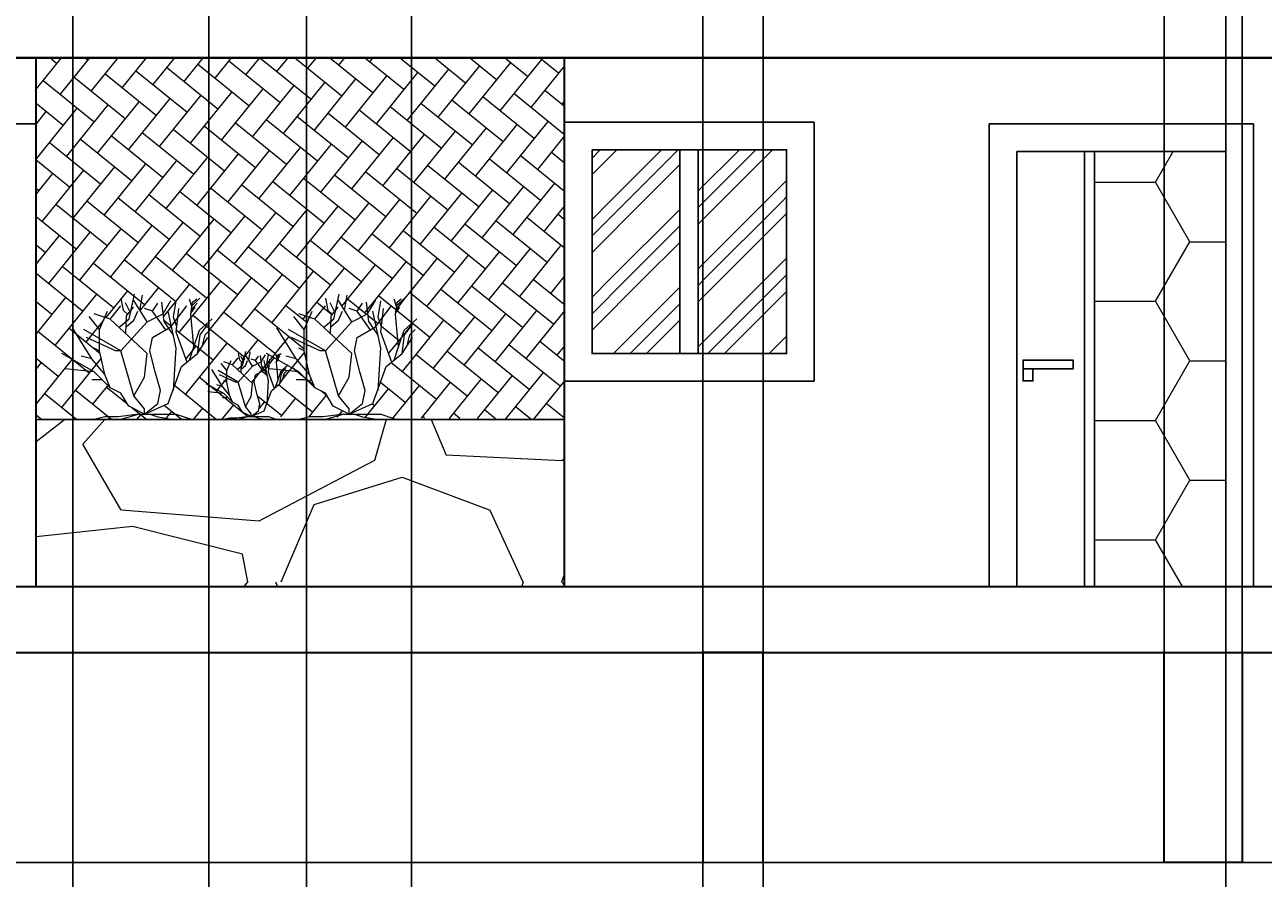
# Model space of a CAD drawing. Units: inches. Extents: x -8 to 554, y -200 to 499.
# Tile 4 of 12: x 214 to 439, y -34 to 121. Entities that reach past the tile are written whole.
import ezdxf

# ---------------------------------------------------------------- set-up
doc = ezdxf.new("R2010")
doc.units = ezdxf.units.IN
doc.header["$MEASUREMENT"] = 0
for name, color, linetype, lineweight in [('A-ANNO-DIMS', 2, 'Continuous', 18), ('A-COLS', 1, 'Continuous', 35), ('A-DOOR', 3, 'Continuous', 25), ('A-DOOR-GATE', 3, 'Continuous', 25), ('A-DOOR-PATT', 252, 'Continuous', 13), ('A-FLOR', 7, 'Continuous', 35), ('A-GLAZ', 4, 'Continuous', 25), ('A-GLAZ-PATT', 252, 'Continuous', 13), ('A-WALL', 7, 'Continuous', 35), ('A-WALL-PATT', 252, 'Continuous', 13), ('A-WALL-PRPT', 7, 'Continuous', 25), ('L-PLNT-TREE', 94, 'Continuous', 13)]:
    doc.layers.add(name, color=color, linetype=linetype, lineweight=lineweight)
doc.styles.get("Standard").update_dxf_attribs({"font": 'arial.ttf'})
doc.dimstyles.get("Standard").update_dxf_attribs({"dimtxt": 0.18, "dimasz": 0.18, "dimexe": 0.18, "dimexo": 0.0625, "dimgap": 0.09, "dimtad": 0, "dimtih": 1, "dimtoh": 1, "dimdec": 4, "dimzin": 0, "dimdsep": 46, "dimtxsty": 'Standard', "dimcen": 0.09, "dimadec": 0, "dimazin": 0, "dimtfac": 1, "dimtdec": 4, "dimtofl": 0, "dimtmove": 0, "dimatfit": 3, "dimfxl": 1, "dimtolj": 1, "dimtzin": 0, "dimarcsym": 0})

# ---------------------------------------------------------------- blocks, each defined once
blk = doc.blocks.new('*U2')
for p, q in [((-11.433, 18.289), (-10.457, 22.749)), ((-9.48, 19.775), (-8.992, 22.592)), ((-14.88, 18.24), (-12.96, 20.64)), ((-12.471, 19.775), (-12.898, 22.044)), ((-11.28, 19.619), (-12.104, 21.184)), ((-11.921, 18.836), (-10.64, 20.401)), ((-8.16, 17.76), (-10.56, 21.6)), ((-7.2, 19.68), (-6.24, 21.12)), ((-5.086, 17.741), (-5.513, 21.34)), ((-5.28, 19.2), (-3.84, 21.6)), ((-3.84, 16.8), (-0.96, 20.64)), ((-3.377, 18.602), (-2.888, 21.575)), ((-0.508, 21.888), (-0.081, 20.558)), ((-0.203, 19.149), (0.102, 21.34)), ((-0.142, 19.384), (0.59, 20.401)), ((-0.02, 20.01), (0.896, 21.105)), ((0.041, 20.714), (1.384, 22.044)), ((0.102, 21.34), (0.835, 21.888)), ((-16.8, 16.32), (-18.72, 18.72)), ((-14.88, 18.24), (-17.76, 19.2)), ((-16.8, 16.32), (-15.36, 19.68)), ((-8.16, 12), (-14.88, 18.24)), ((-13.325, 16.724), (-11.433, 18.289)), ((-11.677, 19.071), (-12.471, 19.775)), ((-12.043, 15.628), (-11.921, 18.836)), ((-11.982, 16.802), (-10.579, 18.054)), ((-10.579, 18.054), (-9.846, 19.697)), ((-7.2, 19.68), (-8.64, 20.16)), ((-8.16, 17.76), (-5.28, 19.2)), ((-4.8, 16.32), (-7.2, 19.68)), ((-2.88, 12.96), (-4.32, 19.68)), ((-2.766, 16.802), (-3.377, 18.602)), ((-2.88, 15.84), (-2.4, 20.16)), ((0.346, 13.203), (-0.203, 19.149)), ((1.323, 16.254), (3.642, 18.289)), ((-18.24, 11.04), (-21.755, 16.655)), ((-12.96, 12.48), (-19.68, 16.32)), ((-16.8, 12.48), (-16.8, 16.32)), ((-12.96, 12.48), (-8.16, 17.76)), ((-7.2, 14.88), (-3.84, 16.8)), ((-3.377, 15.315), (-5.086, 17.819)), ((-0.96, 10.56), (-2.88, 15.84)), ((0.346, 13.203), (1.323, 16.254)), ((1.44, 15.36), (2.88, 17.28)), ((2.4, 15.36), (3.36, 16.32)), ((-13.92, 12.48), (-19.2, 14.88)), ((-7.68, 12.48), (-7.2, 14.88)), ((0.96, 12), (1.44, 15.36)), ((0.96, 12), (2.88, 14.88)), ((1.92, 13.44), (2.4, 15.36)), ((-17.76, 8.64), (-23.663, 11.961)), ((-18.24, 11.04), (-20.16, 11.52)), ((-16.8, 12.48), (-17.76, 12.96)), ((-15.84, 8.16), (-16.8, 12.48)), ((-12.96, 12.48), (-13.92, 12.48)), ((-10.56, 4.32), (-12.96, 12.48)), ((-8.64, 7.68), (-8.16, 12)), ((-6.72, 8.64), (-7.68, 12.48)), ((-3.36, 5.28), (-2.88, 12.96)), ((-1.92, 9.6), (0.96, 12)), ((-0.48, 10.8), (0.346, 13.203)), ((-17.76, 8.64), (-23.128, 9.222)), ((-15.84, 8.16), (-18.24, 11.04)), ((-4.32, 2.88), (-1.92, 9.6)), ((-16.32, 7.2), (-18.24, 7.2)), ((-14.88, 5.76), (-17.76, 8.64)), ((-14.88, 5.76), (-15.84, 8.16)), ((-10.56, 4.32), (-8.64, 7.68)), ((-5.76, 5.28), (-6.72, 8.64)), ((-12.96, 4.8), (-14.88, 5.76)), ((-11.52, 2.4), (-12.96, 4.8)), ((-6.24, 2.88), (-5.76, 5.28)), ((-8.64, 0.96), (-11.52, 2.4)), ((-8.64, 1.92), (-10.56, 4.32)), ((-8.64, 0.96), (-4.32, 2.88)), ((-8.64, 0.96), (-6.24, 2.88)), ((-15.84, 0.48), (-17.76, 0)), ((-13.44, 0.48), (-15.84, 0.48)), ((-9.6, 0.96), (-13.44, 0.48)), ((-9.6, 0.96), (-12.96, 0)), ((-9.6, 0.96), (-7.68, 0.96)), ((-8.64, 0.96), (-8.64, 1.92)), ((-8.64, 0.96), (-2.88, 0.96)), ((-7.68, 0.96), (-6.24, 0.48)), ((-6.24, 0.48), (-3.36, 0)), ((-2.88, 0.96), (0, 0))]:
    blk.add_line(p, q)
blk = doc.blocks.new('DOOR-LEVER-ELEV')
for points in [[(0, 2.19), (9.08, 2.19), (9.08, 3.81), (0, 3.81)], [(0, 2.19), (1.8, 2.19), (1.8, 0), (0, 0)]]:
    blk.add_lwpolyline(points, close=True)
blk = doc.blocks.new('BALCONY-FRONT-96IN')
blk.add_line((0, 30.31), (96, 30.31))
blk.add_lwpolyline([(0, 30.31), (0, 0), (96, 0), (96, 30.31)])
blk = doc.blocks.new('WINDOW-CASING-TWO-LIGHT')
blk.add_lwpolyline([(0, 47.03), (45.36, 47.03), (45.36, 0), (0, 0)], close=True)
blk = doc.blocks.new('*D31')
at = {"layer": 'A-ANNO-DIMS', "color": 0, "lineweight": -2, "transparency": 16777216}
for p, q in [((24.34, 127.42), (24.34, -199.97)), ((453.32, -30.73), (453.32, -199.97)), ((24.52, -199.79), (238.54, -199.79)), ((453.14, -199.79), (239.12, -199.79))]:
    blk.add_line(p, q, dxfattribs=at)
at = {"layer": 'A-ANNO-DIMS', "color": 0, "transparency": 16777216}
for points in [[(24.52, -199.76), (24.52, -199.82), (24.34, -199.79)], [(453.14, -199.76), (453.14, -199.82), (453.32, -199.79)]]:
    blk.add_solid(points, dxfattribs=at)
at = {"layer": 'Defpoints', "color": 0, "transparency": 16777216}
for p in [(24.34, 127.48), (453.32, -30.67), (453.32, -199.79)]:
    blk.add_point(p, dxfattribs=at)
at = {"layer": 'A-ANNO-DIMS', "color": 0, "transparency": 16777216, "insert": (238.83, -199.79), "char_height": 0.18, "attachment_point": 5}
blk.add_mtext('\\A1;429', dxfattribs=at)
blk = doc.blocks.new('*D32')
at = {"layer": 'A-ANNO-DIMS', "color": 0, "lineweight": -2, "transparency": 16777216}
for p, q in [((24.34, 223.42), (24.34, -199.97)), ((444.34, 223.42), (444.34, -199.97)), ((24.52, -199.79), (234.05, -199.79)), ((444.16, -199.79), (234.63, -199.79))]:
    blk.add_line(p, q, dxfattribs=at)
at = {"layer": 'A-ANNO-DIMS', "color": 0, "transparency": 16777216}
for points in [[(24.52, -199.76), (24.52, -199.82), (24.34, -199.79)], [(444.16, -199.76), (444.16, -199.82), (444.34, -199.79)]]:
    blk.add_solid(points, dxfattribs=at)
at = {"layer": 'Defpoints', "color": 0, "transparency": 16777216}
for p in [(24.34, 223.48), (444.34, 223.48), (444.34, -199.79)]:
    blk.add_point(p, dxfattribs=at)
at = {"layer": 'A-ANNO-DIMS', "color": 0, "transparency": 16777216, "insert": (234.34, -199.79), "char_height": 0.18, "attachment_point": 5}
blk.add_mtext('\\A1;420', dxfattribs=at)
blk = doc.blocks.new('*D55')
at = {"layer": 'A-ANNO-DIMS', "color": 0, "lineweight": -2, "transparency": 16777216}
for p, q in [((204.61, -30.61), (204.61, 498.99)), ((204.79, 498.81), (328.57, 498.81)), ((453.14, 498.81), (329.36, 498.81)), ((453.32, -30.61), (453.32, 498.99))]:
    blk.add_line(p, q, dxfattribs=at)
at = {"layer": 'A-ANNO-DIMS', "color": 0, "transparency": 16777216}
for points in [[(204.79, 498.84), (204.79, 498.78), (204.61, 498.81)], [(453.14, 498.84), (453.14, 498.78), (453.32, 498.81)]]:
    blk.add_solid(points, dxfattribs=at)
at = {"layer": 'Defpoints', "color": 0, "transparency": 16777216}
for p in [(453.32, 498.81), (204.61, -30.67), (453.32, -30.67)]:
    blk.add_point(p, dxfattribs=at)
at = {"layer": 'A-ANNO-DIMS', "color": 0, "transparency": 16777216, "insert": (328.96, 498.81), "char_height": 0.18, "attachment_point": 5}
blk.add_mtext('\\A1;248.7', dxfattribs=at)
blk = doc.blocks.new('*D62')
at = {"layer": 'A-ANNO-DIMS', "color": 0, "lineweight": -2, "transparency": 16777216}
for p, q in [((189.3, 7.54), (189.3, 498.99)), ((189.48, 498.81), (263.01, 498.81)), ((337.31, 498.81), (263.78, 498.81)), ((337.49, 7.54), (337.49, 498.99))]:
    blk.add_line(p, q, dxfattribs=at)
at = {"layer": 'A-ANNO-DIMS', "color": 0, "transparency": 16777216}
for points in [[(189.48, 498.84), (189.48, 498.78), (189.3, 498.81)], [(337.31, 498.84), (337.31, 498.78), (337.49, 498.81)]]:
    blk.add_solid(points, dxfattribs=at)
at = {"layer": 'Defpoints', "color": 0, "transparency": 16777216}
for p in [(337.49, 498.81), (189.3, 7.48), (337.49, 7.48)]:
    blk.add_point(p, dxfattribs=at)
at = {"layer": 'A-ANNO-DIMS', "color": 0, "transparency": 16777216, "insert": (263.4, 498.81), "char_height": 0.18, "attachment_point": 5}
blk.add_mtext('\\A1;148.2', dxfattribs=at)
blk = doc.blocks.new('*D63')
at = {"layer": 'A-ANNO-DIMS', "color": 0, "lineweight": -2, "transparency": 16777216}
for p, q in [((337.49, -52.76), (337.49, 498.99)), ((337.67, 498.81), (342.51, 498.81)), ((348.26, 498.81), (343.42, 498.81)), ((348.44, -52.76), (348.44, 498.99))]:
    blk.add_line(p, q, dxfattribs=at)
at = {"layer": 'A-ANNO-DIMS', "color": 0, "transparency": 16777216}
for points in [[(337.67, 498.84), (337.67, 498.78), (337.49, 498.81)], [(348.26, 498.84), (348.26, 498.78), (348.44, 498.81)]]:
    blk.add_solid(points, dxfattribs=at)
at = {"layer": 'Defpoints', "color": 0, "transparency": 16777216}
for p in [(348.44, 498.81), (337.49, -52.82), (348.44, -52.82)]:
    blk.add_point(p, dxfattribs=at)
at = {"layer": 'A-ANNO-DIMS', "color": 0, "transparency": 16777216, "insert": (342.97, 498.81), "char_height": 0.18, "attachment_point": 5}
blk.add_mtext('\\A1;10.946', dxfattribs=at)
blk = doc.blocks.new('*D64')
at = {"layer": 'A-ANNO-DIMS', "color": 0, "lineweight": -2, "transparency": 16777216}
for p, q in [((337.49, 7.54), (337.49, 498.99)), ((337.67, 498.81), (379.02, 498.81)), ((421.13, 498.81), (379.78, 498.81)), ((421.31, 7.54), (421.31, 498.99))]:
    blk.add_line(p, q, dxfattribs=at)
at = {"layer": 'A-ANNO-DIMS', "color": 0, "transparency": 16777216}
for points in [[(337.67, 498.84), (337.67, 498.78), (337.49, 498.81)], [(421.13, 498.84), (421.13, 498.78), (421.31, 498.81)]]:
    blk.add_solid(points, dxfattribs=at)
at = {"layer": 'Defpoints', "color": 0, "transparency": 16777216}
for p in [(421.31, 498.81), (337.49, 7.48), (421.31, 7.48)]:
    blk.add_point(p, dxfattribs=at)
at = {"layer": 'A-ANNO-DIMS', "color": 0, "transparency": 16777216, "insert": (379.4, 498.81), "char_height": 0.18, "attachment_point": 5}
blk.add_mtext('\\A1;83.81', dxfattribs=at)
blk = doc.blocks.new('*D65')
at = {"layer": 'A-ANNO-DIMS', "color": 0, "lineweight": -2, "transparency": 16777216}
for p, q in [((421.31, 7.54), (421.31, 498.99)), ((421.49, 498.81), (428, 498.81)), ((435.29, 498.81), (428.77, 498.81)), ((435.47, 7.54), (435.47, 498.99))]:
    blk.add_line(p, q, dxfattribs=at)
at = {"layer": 'A-ANNO-DIMS', "color": 0, "transparency": 16777216}
for points in [[(421.49, 498.84), (421.49, 498.78), (421.31, 498.81)], [(435.29, 498.84), (435.29, 498.78), (435.47, 498.81)]]:
    blk.add_solid(points, dxfattribs=at)
at = {"layer": 'Defpoints', "color": 0, "transparency": 16777216}
for p in [(435.47, 498.81), (421.31, 7.48), (435.47, 7.48)]:
    blk.add_point(p, dxfattribs=at)
at = {"layer": 'A-ANNO-DIMS', "color": 0, "transparency": 16777216, "insert": (428.39, 498.81), "char_height": 0.18, "attachment_point": 5}
blk.add_mtext('\\A1;14.16', dxfattribs=at)
blk = doc.blocks.new('*D67')
at = {"layer": 'A-ANNO-DIMS', "color": 0, "lineweight": -2, "transparency": 16777216}
for p, q in [((223.01, 427.42), (223.01, -199.97)), ((247.72, 427.42), (247.72, -199.97)), ((223.19, -199.79), (234.9, -199.79)), ((247.54, -199.79), (235.83, -199.79))]:
    blk.add_line(p, q, dxfattribs=at)
at = {"layer": 'A-ANNO-DIMS', "color": 0, "transparency": 16777216}
for points in [[(223.19, -199.76), (223.19, -199.82), (223.01, -199.79)], [(247.54, -199.76), (247.54, -199.82), (247.72, -199.79)]]:
    blk.add_solid(points, dxfattribs=at)
at = {"layer": 'Defpoints', "color": 0, "transparency": 16777216}
for p in [(223.01, 427.48), (247.72, 427.48), (247.72, -199.79)]:
    blk.add_point(p, dxfattribs=at)
at = {"layer": 'A-ANNO-DIMS', "color": 0, "transparency": 16777216, "insert": (235.36, -199.79), "char_height": 0.18, "attachment_point": 5}
blk.add_mtext('\\A1;24.705', dxfattribs=at)
blk = doc.blocks.new('*D68')
at = {"layer": 'A-ANNO-DIMS', "color": 0, "lineweight": -2, "transparency": 16777216}
for p, q in [((247.72, 371.73), (247.72, -199.97)), ((265.46, 371.73), (265.46, -199.97)), ((247.9, -199.79), (256.13, -199.79)), ((265.28, -199.79), (257.04, -199.79))]:
    blk.add_line(p, q, dxfattribs=at)
at = {"layer": 'A-ANNO-DIMS', "color": 0, "transparency": 16777216}
for points in [[(247.9, -199.76), (247.9, -199.82), (247.72, -199.79)], [(265.28, -199.76), (265.28, -199.82), (265.46, -199.79)]]:
    blk.add_solid(points, dxfattribs=at)
at = {"layer": 'Defpoints', "color": 0, "transparency": 16777216}
for p in [(247.72, 371.79), (265.46, 371.79), (265.46, -199.79)]:
    blk.add_point(p, dxfattribs=at)
at = {"layer": 'A-ANNO-DIMS', "color": 0, "transparency": 16777216, "insert": (256.59, -199.79), "char_height": 0.18, "attachment_point": 5}
blk.add_mtext('\\A1;17.744', dxfattribs=at)
blk = doc.blocks.new('*D69')
at = {"layer": 'A-ANNO-DIMS', "color": 0, "lineweight": -2, "transparency": 16777216}
for p, q in [((265.46, 371.73), (265.46, -199.97)), ((284.57, 371.73), (284.57, -199.97)), ((265.64, -199.79), (274.65, -199.79)), ((284.39, -199.79), (275.38, -199.79))]:
    blk.add_line(p, q, dxfattribs=at)
at = {"layer": 'A-ANNO-DIMS', "color": 0, "transparency": 16777216}
for points in [[(265.64, -199.76), (265.64, -199.82), (265.46, -199.79)], [(284.39, -199.76), (284.39, -199.82), (284.57, -199.79)]]:
    blk.add_solid(points, dxfattribs=at)
at = {"layer": 'Defpoints', "color": 0, "transparency": 16777216}
for p in [(265.46, 371.79), (284.57, 371.79), (284.57, -199.79)]:
    blk.add_point(p, dxfattribs=at)
at = {"layer": 'A-ANNO-DIMS', "color": 0, "transparency": 16777216, "insert": (275.01, -199.79), "char_height": 0.18, "attachment_point": 5}
blk.add_mtext('\\A1;19.11', dxfattribs=at)
blk = doc.blocks.new('*D71')
at = {"layer": 'A-ANNO-DIMS', "color": 0, "lineweight": -2, "transparency": 16777216}
for p, q in [((444.34, 439.42), (444.34, -199.97)), ((432.52, 427.42), (432.52, -199.97)), ((432.7, -199.79), (437.97, -199.79)), ((444.16, -199.79), (438.89, -199.79))]:
    blk.add_line(p, q, dxfattribs=at)
at = {"layer": 'A-ANNO-DIMS', "color": 0, "transparency": 16777216}
for points in [[(432.7, -199.76), (432.7, -199.82), (432.52, -199.79)], [(444.16, -199.76), (444.16, -199.82), (444.34, -199.79)]]:
    blk.add_solid(points, dxfattribs=at)
at = {"layer": 'Defpoints', "color": 0, "transparency": 16777216}
for p in [(444.34, 439.48), (432.52, 427.48), (444.34, -199.79)]:
    blk.add_point(p, dxfattribs=at)
at = {"layer": 'A-ANNO-DIMS', "color": 0, "transparency": 16777216, "insert": (438.43, -199.79), "char_height": 0.18, "attachment_point": 5}
blk.add_mtext('\\A1;11.825', dxfattribs=at)

msp = doc.modelspace()

# ---------------------------------------------------------------- hatches: boundary and pattern name
at = {"layer": 'A-DOOR-PATT', "transparency": 33554523}
h = msp.add_hatch(dxfattribs=at)
h.set_pattern_fill('HONEY', color=256, scale=100)
h.set_pattern_definition([(0, (-117.809, -80.312), (18.75, 10.82532), [12.5, -25]), (120, (-117.809, -80.312), (-18.75, 10.82532), [12.5, -25]), (60, (-117.809, -80.312), (4e-15, 21.65064), [-25, 12.5])])
h.paths.add_polyline_path([(211.3421, 314.4814), (187.4809, 314.4814), (187.4809, 235.4814), (211.3421, 235.4814)])
h.paths.add_polyline_path([(211.3421, 206.4814), (187.4809, 206.4814), (187.4809, 127.4814), (211.3421, 127.4814)])
h.paths.add_polyline_path([(211.3421, 98.4814), (187.4809, 98.4814), (187.4809, 19.4814), (211.3421, 19.4814)])
h.paths.add_polyline_path([(432.5174, 98.4814), (408.6562, 98.4814), (408.6562, 19.4814), (432.5174, 19.4814)])
h.paths.add_polyline_path([(432.5174, 206.4814), (408.6562, 206.4814), (408.6562, 127.4814), (432.5174, 127.4814), (432.5174, 155.7921)])
h.paths.add_polyline_path([(432.5174, 314.4814), (408.6562, 314.4814), (408.6562, 235.4814), (432.5174, 235.4814)])
at = {"layer": 'A-GLAZ-PATT'}
h = msp.add_hatch(dxfattribs=at)
h.set_pattern_fill('GOST_GROUND', color=256)
h.set_pattern_definition([(45, (-117.809, -80.312), (14.14214, 0), [20]), (45, (-114.809, -80.312), (14.14214, 0), [20]), (45, (-111.809, -80.312), (14.14214, 0), [20])])
h.paths.add_polyline_path([(83.5906, 206.2713), (71.2048, 206.2713), (71.2048, 187.4661), (83.5906, 187.4661)])
h.paths.add_polyline_path([(95.9765, 187.4661), (83.5906, 187.4661), (83.5906, 168.661), (95.9765, 168.661)])
h.paths.add_polyline_path([(83.5906, 98.2713), (71.2048, 98.2713), (71.2048, 79.4661), (83.5906, 79.4661)])
h.paths.add_polyline_path([(95.9765, 79.4661), (83.5906, 79.4661), (83.5906, 60.661), (95.9765, 60.661)])
h.paths.add_polyline_path([(333.2924, 98.788), (317.3421, 98.788), (317.3421, 61.7623), (333.2924, 61.7623)])
h.paths.add_polyline_path([(352.699, 98.788), (336.6386, 98.788), (336.6386, 61.7623), (352.699, 61.7623)])
h.paths.add_polyline_path([(333.2924, 206.788), (317.3421, 206.788), (317.3421, 169.7623), (333.2924, 169.7623)])
h.paths.add_polyline_path([(352.699, 206.788), (336.6386, 206.788), (336.6386, 169.7623), (352.699, 169.7623)])
h.paths.add_polyline_path([(333.2924, 314.788), (317.3421, 314.788), (317.3421, 277.7623), (333.2924, 277.7623)])
h.paths.add_polyline_path([(352.699, 314.788), (336.6386, 314.788), (336.6386, 277.7623), (352.699, 277.7623)])
h.paths.add_polyline_path([(95.9765, 295.4661), (83.5906, 295.4661), (83.5906, 276.661), (95.9765, 276.661)])
h.paths.add_polyline_path([(83.5906, 314.2713), (71.2048, 314.2713), (71.2048, 295.4661), (83.5906, 295.4661)])
at = {"layer": 'A-WALL-PATT'}
h = msp.add_hatch(dxfattribs=at)
h.set_pattern_fill('GRAVEL', color=256, scale=100)
h.set_pattern_definition([(228.0128, (-45.809, 19.688), (-800, -900), [13.4536, -1331.909]), (184.9697, (-54.8087, 9.688), (1200, 100), [23.0868, -2285.5925]), (132.5104, (-77.809, 7.688), (1000, -1100), [16.279, -1611.6033]), (267.2737, (-116.8087, -17.312), (100, 2000), [21.0238, -2081.3558]), (292.83365, (-117.8087, -38.312), (-500, 1200), [20.6155, -2040.9373]), (357.2737, (-109.8087, -57.312), (-2000, 100), [21.0238, -2081.3558]), (37.69424, (-88.8087, -58.3118), (-1300, -1000), [27.803, -2752.4849]), (72.2553, (-66.8087, -41.312), (700, 2200), [26.2488, -2598.632]), (121.4296, (-58.8087, -16.312), (-800, 1300), [21.095, -2088.4073]), (175.2364, (-69.809, 1.688), (1100, -100), [24.083, -1180.076]), (222.39744, (-93.8087, 3.6882), (-1200, -1100), [31.1448, -3083.3375]), (138.814, (-17.809, -18.312), (-700, 600), [10.63, -1052.3845]), (171.4692, (-25.8087, -11.312), (1300, -200), [20.2237, -2002.151]), (225, (-45.81, -8.31), (-1e-14, -100), [14.142, -127.279]), (203.1986, (-52.809, 3.688), (500, 200), [7.616, -753.9615]), (291.8014, (-59.809, 0.688), (-100, 300), [10.77, -527.746]), (30.9638, (-55.809, -9.312), (300, 200), [17.493, -565.602]), (161.565, (-40.81, -0.312), (200, -100), [12.649, -303.579]), (16.3895, (-117.8087, 0.688), (1000, 300), [17.72, -1754.2845]), (70.3462, (-100.809, 5.688), (-400, -1100), [14.866, -1471.741]), (293.1986, (-40.809, 19.688), (-200, 500), [15.2315, -746.346]), (343.6105, (-34.8087, 5.688), (-1000, 300), [17.72, -1754.2845]), (339.444, (-117.809, -61.312), (-500, 200), [17.088, -837.3124]), (294.7751, (-101.809, -67.312), (-500, 1100), [14.318, -1417.4643]), (66.8014, (-39.809, -80.312), (200, 500), [15.2315, -746.346]), (17.354, (-33.809, -66.312), (-1300, -400), [16.763, -1659.5424]), (69.444, (-88.809, -80.312), (-200, -500), [8.544, -845.8564]), (101.31, (-45.809, -80.312), (-100, 400), [5.099, -504.803]), (165.9638, (-46.809, -75.312), (300, -100), [20.6155, -391.695]), (186.009, (-66.8087, -70.312), (1000, 100), [19.105, -1891.3923]), (303.69, (-55.81, -18.312), (-100, 200), [14.422, -346.133]), (353.1572, (-47.8087, -30.312), (1700, -200), [25.1794, -2492.7563]), (60.9454, (-22.809, -33.312), (-400, -700), [10.2956, -1019.2674]), (90, (-17.81, -24.31), (-100, 100), [6, -94]), (120.2564, (-68.809, -67.312), (400, -700), [13.8924, -1375.352]), (48.0128, (-75.809, -55.312), (800, 900), [26.907, -1318.455]), (0, (-57.81, -35.31), (100, 100), [26, -74]), (325.3048, (-31.809, -35.312), (1000, -700), [15.8114, -1565.3274]), (254.0546, (-18.809, -44.312), (-100, -400), [14.56, -713.451]), (207.646, (-22.8087, -58.312), (-1900, -1000), [23.7065, -2346.9474]), (175.4261, (-43.8087, -69.312), (-1300, 100), [25.08, -2482.9073])])
h.paths.add_polyline_path([(48.6882, -52.5186), (24.3421, -52.5186), (24.3421, -112.5186), (48.6882, -112.5186)])
h.paths.add_polyline_path([(212.2282, -52.5186), (140.2282, -52.5186), (128.2282, -52.5186), (128.2282, -112.5186), (140.2282, -112.5186), (140.2282, -64.9665), (202.9211, -64.9665), (202.9211, -112.5186), (212.2282, -112.5186)])
h.paths.add_polyline_path([(312.3421, 49.7921), (216.3421, 49.7921), (216.3421, 19.4814), (312.3421, 19.4814)])
h.paths.add_polyline_path([(312.3421, 157.7921), (216.3421, 157.7921), (216.3421, 127.4814), (312.3421, 127.4814)])
h.paths.add_polyline_path([(312.3421, 265.7921), (216.3421, 265.7921), (216.3421, 235.4814), (312.3421, 235.4814)])
h.paths.add_polyline_path([(432.5174, 371.7921), (215.6778, 371.7921), (215.6778, 368.5162), (215.6778, 357.6367), (35.7874, 357.6367), (35.7874, 360.9127), (35.7874, 371.7921), (24.3421, 371.7921), (24.3421, 343.4814), (35.7874, 343.4814), (432.5174, 343.4814)])
at = {"layer": 'A-WALL-PATT', "transparency": 33554569}
h = msp.add_hatch(dxfattribs=at)
h.set_pattern_fill('AR-HBONE', color=256, angle=96)
h.set_pattern_definition([(141, (-117.8087, -80.312), (-5.625865, -0.591302), [12, -4]), (231, (-120.9173, -77.7945), (-5.625865, -0.591302), [12, -4])])
h.paths.add_polyline_path([(312.3421, 115.4814), (216.3421, 115.4814), (216.3421, 49.7921), (250.4667, 49.7921), (251.5112, 50.0532), (252.8169, 50.0532), (255.3238, 50.3666), (253.8614, 51.0978), (253.078, 52.4035), (252.0335, 52.9257), (251.5112, 54.2314), (250.9889, 56.5816), (250.9889, 58.6707), (251.5112, 59.8894), (252.0335, 59.7153), (253.4528, 61.4895), (253.992, 60.4655), (254.0945, 60.5908), (253.9087, 59.7419), (253.623, 59.5055), (253.5764, 58.2825), (256.1145, 55.9258), (256.4728, 54.4925), (256.995, 52.6646), (256.632, 50.8494), (255.6521, 50.4139), (255.9505, 50.3144), (258.5619, 50.3144), (312.3421, 49.7921)])
h.paths.add_polyline_path([(260.0854, 60.6921), (260.1153, 60.6752), (260.163, 60.7322), (260.1127, 60.8887)], flags=16)
h.paths.add_polyline_path([(270.7709, 69.6415), (271.1925, 71.568), (273.7025, 67.5521), (276.5825, 68.9921), (276.5999, 69.0212), (276.7653, 67.6275), (277.6264, 66.3658), (278.0225, 66.5921), (279.2746, 68.2617), (278.9825, 65.6321), (280.9471, 60.2293), (281.3825, 60.5921), (282.2085, 62.9951), (281.6472, 69.0743), (281.6854, 69.1274), (281.8332, 70.189), (281.7729, 70.3768), (281.8731, 70.4761), (281.6595, 68.9411), (282.2085, 62.9951), (281.3825, 60.5921), (279.9425, 59.3921), (277.5425, 52.6721), (273.2225, 50.7521), (270.3425, 52.1921), (268.9025, 54.5921), (266.9825, 55.5521), (264.1025, 58.4321), (261.9512, 58.6653), (261.4344, 58.1484), (261.1732, 57.1039), (260.6509, 56.3205), (259.0841, 55.0148), (258.3126, 52.8545), (258.5619, 56.8428), (258.2854, 58.1328), (257.8241, 58.8087), (257.5362, 58.6442), (256.624, 59.9214), (257.2562, 60.2375), (257.2657, 60.2534), (257.3556, 59.4952), (257.8241, 58.8087), (258.0396, 58.9319), (258.7208, 59.8402), (258.6303, 59.0254), (264.1025, 58.4321), (266.9825, 55.5521), (266.0225, 57.9521), (265.0625, 62.2721), (265.0625, 66.1121), (266.0225, 68.3521), (266.9825, 68.0321), (268.5785, 66.5501), (269.9041, 67.6466), (269.9415, 68.6281)], flags=16)
h.paths.add_polyline_path([(244.6939, 70.4761), (244.4802, 68.9411), (245.0292, 62.9951), (244.2032, 60.5921), (242.7632, 59.3921), (240.3632, 52.6721), (236.0432, 50.7521), (233.1632, 52.1921), (231.7232, 54.5921), (229.8032, 55.5521), (228.8432, 57.9521), (227.8832, 62.2721), (227.8832, 66.1121), (228.8432, 68.3521), (229.8032, 68.0321), (231.3992, 66.5501), (232.7249, 67.6466), (232.7622, 68.6281), (233.5916, 69.6415), (234.0132, 71.568), (236.5232, 67.5521), (239.4032, 68.9921), (239.4206, 69.0212), (239.586, 67.6275), (240.4471, 66.3658), (240.8432, 66.5921), (242.0954, 68.2617), (241.8032, 65.6321), (243.7678, 60.2293), (244.2032, 60.5921), (245.0292, 62.9951), (244.4679, 69.0743), (244.5061, 69.1274), (244.6539, 70.189), (244.5936, 70.3768)], flags=16)
h.paths.add_polyline_path([(312.3421, 223.4814), (216.3421, 223.4814), (216.3421, 157.7921), (312.3421, 157.7921)])
h.paths.add_polyline_path([(260.0854, 168.6921), (260.1153, 168.6752), (260.163, 168.7322), (260.1127, 168.8887)], flags=16)
h.paths.add_polyline_path([(271.1925, 179.568), (273.7025, 175.5521), (276.5825, 176.9921), (276.5999, 177.0212), (276.7653, 175.6275), (277.6264, 174.3658), (278.0225, 174.5921), (279.2746, 176.2617), (278.9825, 173.6321), (280.9471, 168.2293), (281.3825, 168.5921), (282.2085, 170.9951), (281.6472, 177.0743), (281.6854, 177.1274), (281.8332, 178.189), (281.7729, 178.3768), (281.8731, 178.4761), (281.6595, 176.9411), (282.2085, 170.9951), (281.3825, 168.5921), (279.9425, 167.3921), (277.5425, 160.6721), (273.2225, 158.7521), (270.3425, 160.1921), (268.9025, 162.5921), (266.9825, 163.5521), (264.1025, 166.4321), (261.9512, 166.6653), (261.4344, 166.1484), (261.1732, 165.1039), (260.6509, 164.3205), (259.0841, 163.0148), (257.7785, 159.3589), (255.6521, 158.4139), (255.9505, 158.3144), (255.4282, 158.3144), (253.8614, 159.0978), (253.078, 160.4035), (252.0335, 160.9257), (251.5112, 162.2314), (250.9889, 164.5816), (250.9889, 166.6707), (251.5112, 167.8894), (252.0335, 167.7153), (253.2217, 169.2005), (253.344, 168.5504), (253.7597, 168.1818), (254.0945, 168.5908), (254.3239, 169.6389), (255.6894, 167.4541), (257.2562, 168.2375), (257.2657, 168.2534), (257.3556, 167.4952), (257.8241, 166.8087), (258.0396, 166.9319), (258.7208, 167.8402), (258.6303, 167.0254), (264.1025, 166.4321), (266.9825, 163.5521), (266.0225, 165.9521), (265.0625, 170.2721), (265.0625, 174.1121), (266.0225, 176.3521), (266.9825, 176.0321), (268.5785, 174.5501), (269.9041, 175.6466), (269.9415, 176.6281), (270.7709, 177.6415)], flags=16)
h.paths.add_polyline_path([(253.5764, 166.2825), (255.6894, 164.3205), (255.4282, 161.9703), (254.3837, 160.1423), (253.078, 164.5816), (254.1446, 165.7549), (252.9018, 166.909), (253.623, 167.5055)], flags=0)
h.paths.add_polyline_path([(245.0292, 170.9951), (244.2032, 168.5921), (242.7632, 167.3921), (240.3632, 160.6721), (236.0432, 158.7521), (233.1632, 160.1921), (231.7232, 162.5921), (229.8032, 163.5521), (228.8432, 165.9521), (227.8832, 170.2721), (227.8832, 174.1121), (228.8432, 176.3521), (229.8032, 176.0321), (231.3992, 174.5501), (232.7249, 175.6466), (232.7622, 176.6281), (233.5916, 177.6415), (234.0132, 179.568), (236.5232, 175.5521), (239.4032, 176.9921), (239.4206, 177.0212), (239.586, 175.6275), (240.4471, 174.3658), (240.8432, 174.5921), (242.0954, 176.2617), (241.8032, 173.6321), (243.7678, 168.2293), (244.2032, 168.5921), (245.0292, 170.9951), (244.4679, 177.0743), (244.5061, 177.1274), (244.6539, 178.189), (244.5936, 178.3768), (244.6939, 178.4761), (244.4802, 176.9411)], flags=16)
h.paths.add_polyline_path([(312.3421, 331.4814), (216.3421, 331.4814), (216.3421, 265.7921), (312.3421, 265.7921)])
h.paths.add_polyline_path([(260.0854, 276.6921), (260.1153, 276.6752), (260.163, 276.7322), (260.1127, 276.8887)], flags=16)
h.paths.add_polyline_path([(281.8731, 286.4761), (281.6595, 284.9411), (282.2085, 278.9951), (281.3825, 276.5921), (279.9425, 275.3921), (277.5425, 268.6721), (273.2225, 266.7521), (270.3425, 268.1921), (268.9025, 270.5921), (266.9825, 271.5521), (264.1025, 274.4321), (261.9512, 274.6653), (261.4344, 274.1484), (261.1732, 273.1039), (260.6509, 272.3205), (259.0841, 271.0148), (257.7785, 267.3589), (255.6521, 266.4139), (255.9505, 266.3144), (255.4282, 266.3144), (253.8614, 267.0978), (253.078, 268.4035), (252.0335, 268.9257), (251.5112, 270.2314), (250.9889, 272.5816), (250.9889, 274.6707), (251.5112, 275.8894), (252.0335, 275.7153), (253.2217, 277.2005), (253.344, 276.5504), (253.7597, 276.1818), (254.0945, 276.5908), (254.3239, 277.6389), (255.6894, 275.4541), (257.2562, 276.2375), (257.2657, 276.2534), (257.3556, 275.4952), (257.8241, 274.8087), (258.0396, 274.9319), (258.7208, 275.8402), (258.6303, 275.0254), (264.1025, 274.4321), (266.9825, 271.5521), (266.0225, 273.9521), (265.0625, 278.2721), (265.0625, 282.1121), (266.0225, 284.3521), (266.9825, 284.0321), (268.5785, 282.5501), (269.9041, 283.6466), (269.9415, 284.6281), (270.7709, 285.6415), (271.1925, 287.568), (273.7025, 283.5521), (276.5825, 284.9921), (276.5999, 285.0212), (276.7653, 283.6275), (277.6264, 282.3658), (278.0225, 282.5921), (279.2746, 284.2617), (278.9825, 281.6321), (280.9471, 276.2293), (281.3825, 276.5921), (282.2085, 278.9951), (281.6472, 285.0743), (281.6854, 285.1274), (281.8332, 286.189), (281.7729, 286.3768)], flags=16)
h.paths.add_polyline_path([(255.6894, 272.3205), (255.4282, 269.9703), (254.3837, 268.1423), (253.078, 272.5816), (254.1446, 273.7549), (252.9018, 274.909), (253.623, 275.5055), (253.5764, 274.2825)], flags=0)
h.paths.add_polyline_path([(245.0292, 278.9951), (244.2032, 276.5921), (242.7632, 275.3921), (240.3632, 268.6721), (236.0432, 266.7521), (233.1632, 268.1921), (231.7232, 270.5921), (229.8032, 271.5521), (228.8432, 273.9521), (227.8832, 278.2721), (227.8832, 282.1121), (228.8432, 284.3521), (229.8032, 284.0321), (231.3992, 282.5501), (232.7249, 283.6466), (232.7622, 284.6281), (233.5916, 285.6415), (234.0132, 287.568), (236.5232, 283.5521), (239.4032, 284.9921), (239.4206, 285.0212), (239.586, 283.6275), (240.4471, 282.3658), (240.8432, 282.5921), (242.0954, 284.2617), (241.8032, 281.6321), (243.7678, 276.2293), (244.2032, 276.5921), (245.0292, 278.9951), (244.4679, 285.0743), (244.5061, 285.1274), (244.6539, 286.189), (244.5936, 286.3768), (244.6939, 286.4761), (244.4802, 284.9411)], flags=16)

# ---------------------------------------------------------------- linework, layer by layer
at = {"layer": 'A-COLS'}
msp.add_lwpolyline([(348.4381, -30.6677), (348.4381, 7.4814), (337.4923, 7.4814), (337.4923, -30.6677)], dxfattribs=at)
msp.add_lwpolyline([(435.4655, -30.6677), (421.3053, -30.6677), (421.3053, 7.4814), (435.4655, 7.4814)], close=True, dxfattribs=at)
at = {"layer": 'A-DOOR'}
for p, q in [((394.5174, 19.4814), (394.5174, 98.4814)), ((394.5174, 98.4814), (432.5174, 98.4814)), ((432.5174, 98.4814), (432.5174, 19.4814))]:
    msp.add_line(p, q, dxfattribs=at)
for points in [[(216.3421, 19.4814), (168.3421, 19.4814), (168.3421, 103.4814), (216.3421, 103.4814)], [(437.5174, 19.4814), (389.5174, 19.4814), (389.5174, 103.4814), (437.5174, 103.4814)], [(406.8193, 98.4814), (408.6562, 98.4814), (408.6562, 19.4814), (406.8193, 19.4814)]]:
    msp.add_lwpolyline(points, close=True, dxfattribs=at)
at = {"layer": 'A-DOOR-GATE'}
msp.add_lwpolyline([(446.0855, -36.3739), (453.3222, -36.3739), (453.3222, -30.6677), (204.6055, -30.6677), (204.6055, -36.3739), (212.2282, -36.3739)], dxfattribs=at)
at = {"layer": 'A-FLOR'}
for p, q in [((24.3421, 115.4814), (444.3421, 115.4814)), ((444.3421, 115.4814), (36.3421, 115.4814)), ((36.3421, 19.4814), (444.3421, 19.4814)), ((24.3421, 7.4814), (444.3421, 7.4814))]:
    msp.add_line(p, q, dxfattribs=at)
at = {"layer": 'A-GLAZ'}
for points in [[(317.3421, 98.788), (352.699, 98.788), (352.699, 61.7623), (317.3421, 61.7623)], [(333.2924, 98.788), (336.6386, 98.788), (336.6386, 61.7623), (333.2924, 61.7623)]]:
    msp.add_lwpolyline(points, close=True, dxfattribs=at)
at = {"layer": 'A-WALL'}
for p, q in [((216.3421, 19.4814), (216.3421, 115.4814)), ((312.3421, 19.4814), (312.3421, 115.4814))]:
    msp.add_line(p, q, dxfattribs=at)

# ---------------------------------------------------------------- block references
at = {"layer": 'A-DOOR'}
msp.add_blockref('DOOR-LEVER-ELEV', (395.6515, 56.7884), dxfattribs=at)
at = {"layer": 'A-GLAZ'}
msp.add_blockref('WINDOW-CASING-TWO-LIGHT', (312.3421, 56.7623), dxfattribs=at)
at = {"layer": 'A-WALL-PRPT'}
msp.add_blockref('BALCONY-FRONT-96IN', (216.3421, 19.4814), dxfattribs=at)
at = {"layer": 'L-PLNT-TREE'}
for p in [(244.6832, 49.7921), (281.8625, 49.7921)]:
    msp.add_blockref('*U2', p, dxfattribs=at)
at = {"layer": 'L-PLNT-TREE', "xscale": 0.5440329233585479, "yscale": 0.5440329233585479, "zscale": 0.5440329233585479}
msp.add_blockref('*U2', (260.1287, 49.7921), dxfattribs=at)

# ---------------------------------------------------------------- dimensions: what is measured, and where the dimension line sits
at = {"layer": 'A-ANNO-DIMS'}
for base, p1, p2, override, picture, middle in [((337.4923, 498.8091), (189.3049, 7.4814), (337.4923, 7.4814), {"dimdec": 1, "dimlfac": 1, "dimrnd": 0, "dimzin": 0, "dimdsep": 46, "dimlunit": 2}, '*D62', (263.3986, 498.8091)), ((453.3222, 498.8091), (204.6055, -30.6677), (453.3222, -30.6677), {"dimdec": 1, "dimlfac": 1, "dimrnd": 0, "dimzin": 0, "dimdsep": 46, "dimlunit": 2}, '*D55', (328.9639, 498.8091)), ((348.4381, 498.8091), (337.4923, -52.8231), (348.4381, -52.8231), {"dimdec": 3, "dimlfac": 1, "dimrnd": 0, "dimzin": 0, "dimdsep": 46, "dimlunit": 2}, '*D63', (342.9652, 498.8091)), ((421.3053, 498.8091), (337.4923, 7.4814), (421.3053, 7.4814), {"dimdec": 2, "dimlfac": 1, "dimrnd": 0, "dimzin": 0, "dimdsep": 46, "dimlunit": 2}, '*D64', (379.3988, 498.8091)), ((435.4655, 498.8091), (421.3053, 7.4814), (435.4655, 7.4814), {"dimdec": 2, "dimlfac": 1, "dimrnd": 0, "dimzin": 0, "dimdsep": 46, "dimlunit": 2}, '*D65', (428.3854, 498.8091)), ((444.3421, -199.7912), (432.5174, 427.4814), (444.3421, 439.4814), {"dimdec": 3, "dimlfac": 1, "dimrnd": 0, "dimzin": 0, "dimdsep": 46, "dimlunit": 2}, '*D71', (438.4297, -199.7912)), ((247.71587, -199.79119), (223.01039, 427.48136), (247.71587, 427.48136), {"dimdec": 3, "dimlfac": 1, "dimrnd": 0, "dimzin": 0, "dimdsep": 46, "dimlunit": 2}, '*D67', (235.36313, -199.79119)), ((265.4598, -199.7912), (247.7159, 371.7921), (265.4598, 371.7921), {"dimdec": 3, "dimlfac": 1, "dimrnd": 0, "dimzin": 0, "dimdsep": 46, "dimlunit": 2}, '*D68', (256.5878, -199.7912)), ((284.5686, -199.7912), (265.4598, 371.7921), (284.5686, 371.7921), {"dimdec": 2, "dimlfac": 1, "dimrnd": 0, "dimzin": 0, "dimdsep": 46, "dimlunit": 2}, '*D69', (275.0142, -199.7912)), ((444.3421, -199.7912), (24.3421, 223.4814), (444.3421, 223.4814), {"dimdec": 0, "dimlfac": 1, "dimrnd": 0, "dimzin": 0, "dimdsep": 46, "dimlunit": 2}, '*D32', (234.3421, -199.7912)), ((453.3222, -199.7912), (24.3421, 127.4814), (453.3222, -30.6677), {"dimdec": 0, "dimlfac": 1, "dimrnd": 0, "dimzin": 0, "dimdsep": 46, "dimlunit": 2}, '*D31', (238.8321, -199.7912))]:
    dim = msp.add_linear_dim(base=base, p1=p1, p2=p2, dimstyle='Standard', override=override, dxfattribs=at)
    dim.commit()
    dim.dimension.update_dxf_attribs({"geometry": picture, "text_midpoint": middle})

doc.saveas('drawing.dxf')
